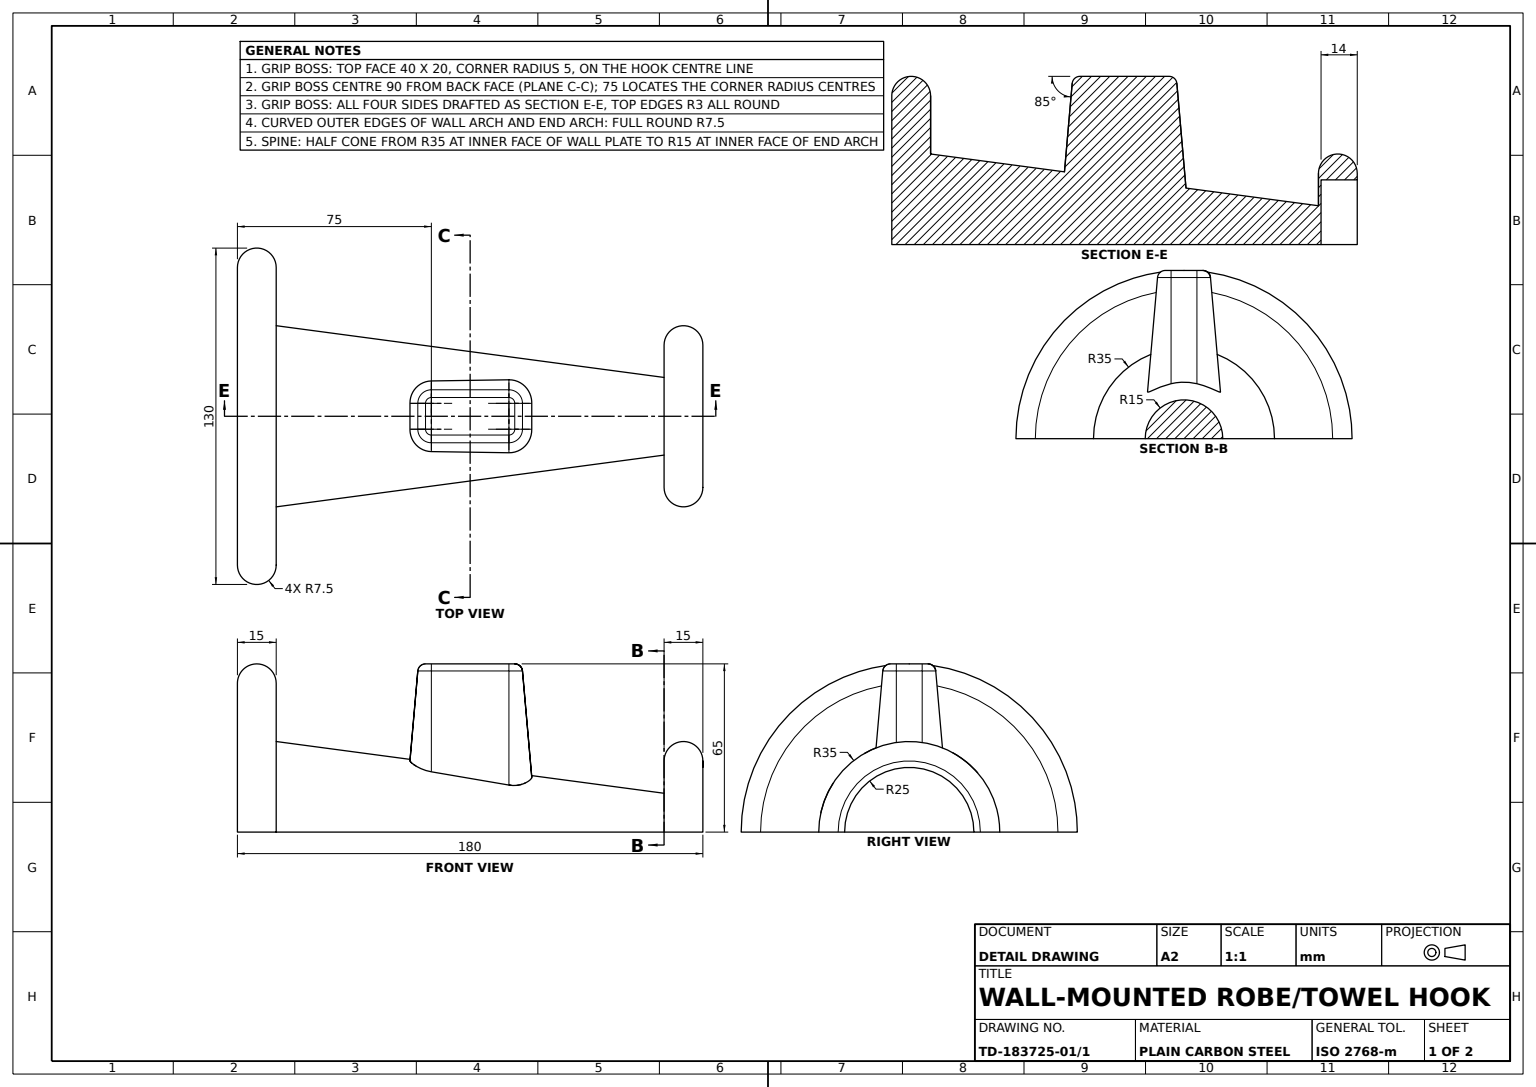
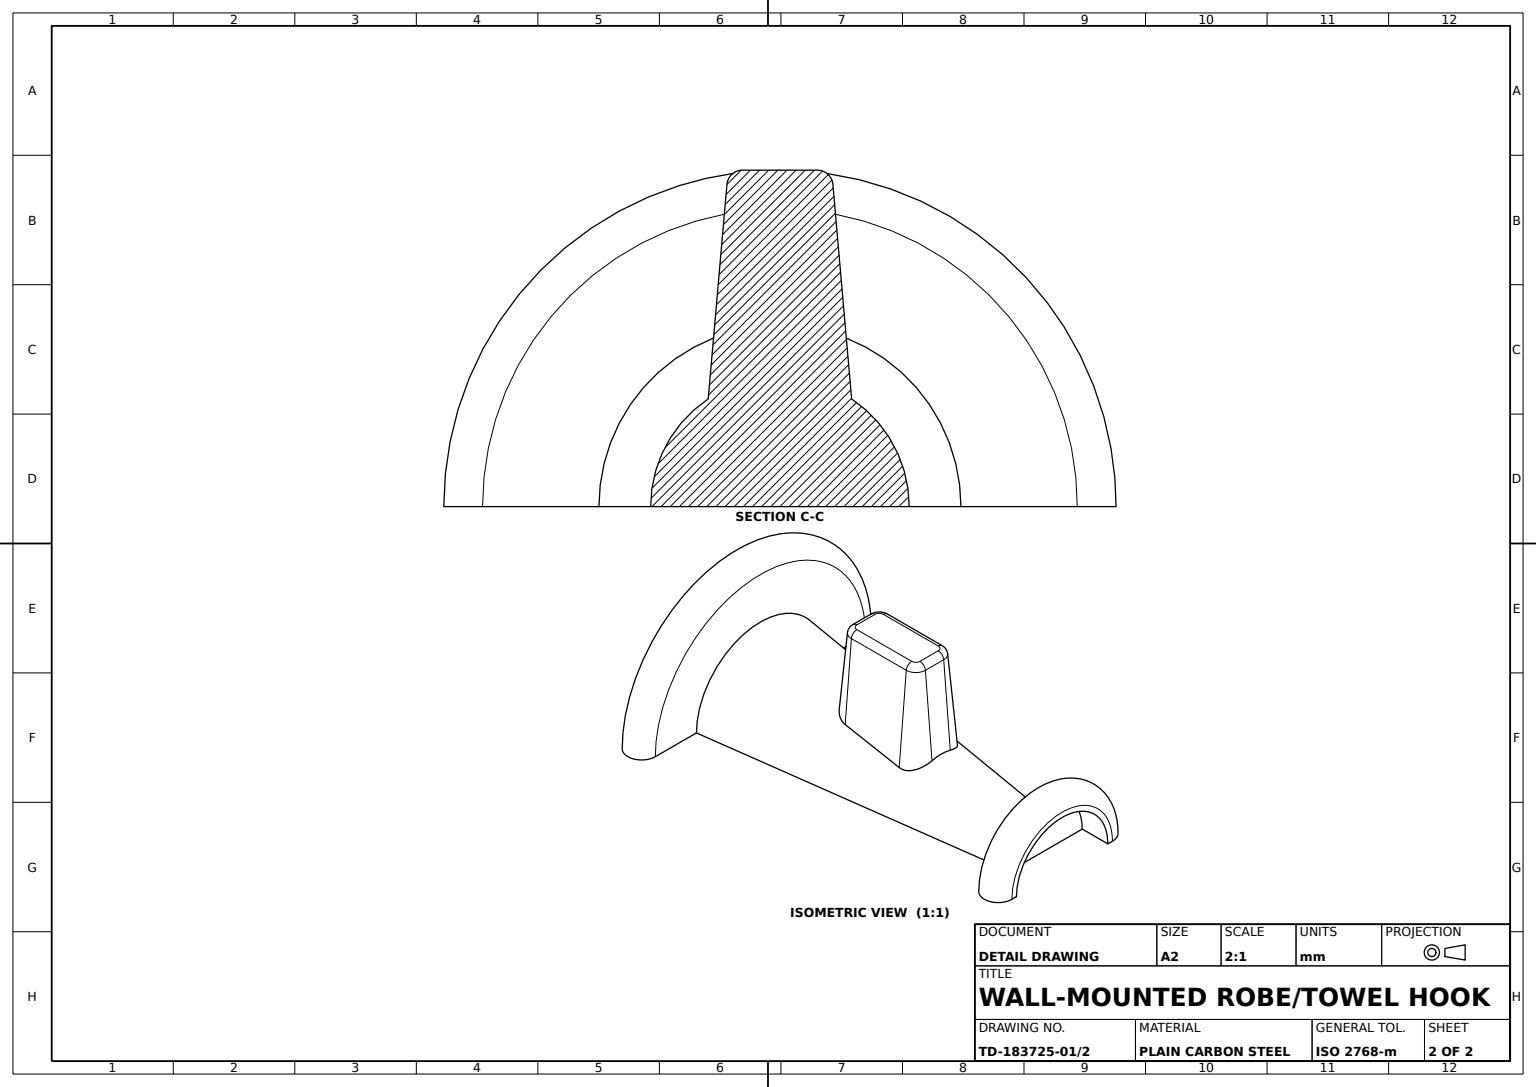
SolidWorks part; units mm, degrees
material "Plain Carbon Steel"
ref_plane "Front Plane" through (0, 0, 0) normal (0, 0, 1) x (1, 0, 0)
ref_plane "Top Plane" through (0, 0, 0) normal (0, 1, 0) x (1, 0, 0)
ref_plane "Right Plane" through (0, 0, 0) normal (1, 0, 0) x (0, 0, -1)
sketch "Hook Body Profile" plane through (0, 0, 0) normal (0, 0, 1) x (1, 0, 0)
  line L0 (0, 0) -> (-90, 0)
  line L1 (0, 0) -> (90, 0)
  line L2 (-90, 0) -> (-90, 57.5)
  line L3 (-75, 0) -> (-75, 57.5)
  line L4 (-75, 57.5) -> (-75, 35)
  line L5 (90, 0) -> (90, 27.5)
  line L6 (75, 0) -> (75, 27.5)
  line L7 (75, 27.5) -> (75, 15)
  line L8 (75, 0) -> (75, 35) construction
  line L9 (-90, 0) -> (-90, 65) construction
  line L10 (-75, 0) -> (-75, 65) construction
  line L11 (90, 0) -> (90, 35) construction
  line L12 (-75, 35) -> (75, 15)
  arc A0 (-75, 57.5) -> (-90, 57.5) centre (-82.5, 57.5) ccw
  arc A1 (90, 27.5) -> (75, 27.5) centre (82.5, 27.5) ccw
  dimension "D1" = 90
  dimension "D2" = 90
  dimension "D3" = 22.5
  dimension "D5" = 12.5
  dimension "D7" = 57.5
  dimension "D8" = 27.5
  dimension "D4" = 15
  dimension "D6" = 15
revolve "Hook Body Revolve" add sketch "Hook Body Profile" angle 360 about L1
sketch "Half Split Cut Sketch" plane through (0, 0, 0) normal (0, 0, 1) x (1, 0, 0)
  line L0 (-118.5158, 0) -> (115.1053, 0)
  line L1 (115.1053, 0) -> (115.1053, -71.9053)
  line L2 (115.1053, -71.9053) -> (-118.5158, -71.9053)
  line L3 (-118.5158, -71.9053) -> (-118.5158, 0)
  dimension "D1" = 233.6211
  dimension "D2" = 71.9053
  dimension "D3" = 115.1053
extrude "Half Split Cut" cut sketch "Half Split Cut Sketch" against normal blind 80 and the other way blind 94
sketch "Boss Plane Offset Line 65" plane through (0, 0, 0) normal (0, 0, 1) x (1, 0, 0)
  line L0 (0, 0) -> (0, 65)
  dimension "D1" = 65
ref_plane "Grip Boss Plane" through (0, 65, 0) normal (0, 1, 0) x (1, 0, 0)
sketch "Grip Boss Sketch 40x20" plane through (0, 65, 0) normal (0, 1, 0) x (1, 0, 0)
  line L1 (-15, 10) -> (15, 10)
  line L2 (-20, 5) -> (-20, -5)
  line L3 (-15, -10) -> (15, -10)
  line L4 (20, 5) -> (20, -5)
  line L5 (-20, 10) -> (20, -10) construction
  line L6 (-20, -10) -> (20, 10) construction
  arc A0 (15, 10) -> (20, 5) centre (15, 5) cw
  arc A1 (15, -10) -> (20, -5) centre (15, -5) ccw
  arc A2 (-20, -5) -> (-15, -10) centre (-15, -5) ccw
  arc A3 (-15, 10) -> (-20, 5) centre (-15, 5) ccw
  point P0 (0, 0)
  dimension "D3" = 5
  dimension "D1" = 40
  dimension "D2" = 20
extrude "Grip Boss Drafted 5deg" add sketch "Grip Boss Sketch 40x20" against normal up to surface (65 mm away) draft 5
fillet "Grip Boss Fillet R3" radius 3 8 edges at (18.5355, 65, 8.5355) (0, 65, 10) (-18.5355, 65, 8.5355) (-20, 65, 0) (-18.5355, 65, -8.5355) (0, 65, -10) (18.5355, 65, -8.5355) (20, 65, 0)
sketch "Hook End Recess Sketch Ø50" plane through (90, 0, 0) normal (1, 0, 0) x (0, 0, -1)
  circle A0 centre (0, 0) radius 25
  dimension "D1" = 50
extrude "Hook End Recess Ø50x14" cut sketch "Hook End Recess Sketch Ø50" against normal blind 14
